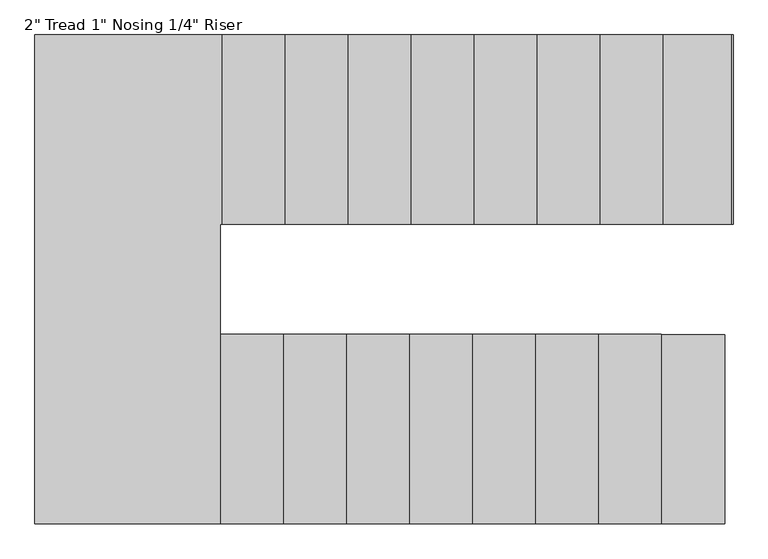
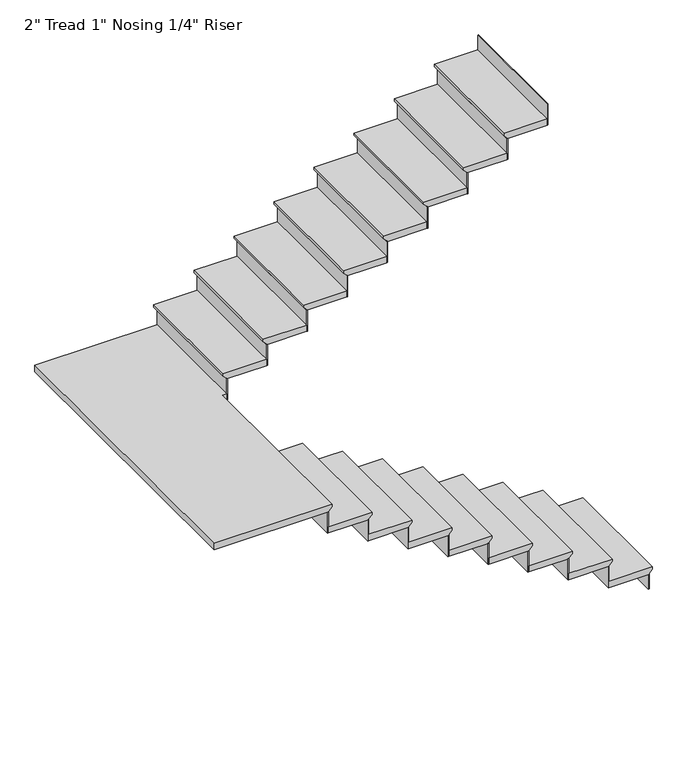
"""IFC4 building model written with IfcOpenShell, lengths in millimetres: stair flight geometry."""

from ifc_helpers import new_model, si_unit, origin, place, context, project, spatial, faceted_brep, source, transform, mapped, element, save


def stair_flight_1ef6648f(model_context):
    return source(origin(), model_context, "Body", "Brep", [
        faceted_brep([(-7930.9736584, -7547.2396616, 455.0833333), (-7930.9736584, -7547.2396616, 474.1333333), (-7930.9736584, -8461.6396616, 474.1333333), (-7930.9736584, -8461.6396616, 455.0833333), (-7956.3736584, -7547.2396616, 429.6833333), (-7956.3736584, -8461.6396616, 429.6833333), (-8261.1736584, -7547.2396616, 474.1333333), (-8261.1736584, -8461.6396616, 474.1333333), (-7956.3736584, -8461.6396616, 423.3333333), (-8261.1736584, -8461.6396616, 423.3333333), (-8261.1736584, -7547.2396616, 423.3333333), (-7956.3736584, -7547.2396616, 423.3333333)], [[[0, 1, 2, 3]], [[4, 0, 3, 5]], [[2, 1, 6, 7]], [[8, 9, 10, 11]], [[2, 7, 9, 8, 5, 3]], [[8, 11, 4, 5]], [[6, 1, 0, 4, 11, 10]], [[7, 6, 10, 9]]]),
        faceted_brep([(-7956.3736584, -7547.2396616, 423.3333333), (-7956.3736584, -7547.2396616, 304.8), (-7962.7236584, -7547.2396616, 304.8), (-7962.7236584, -7547.2396616, 423.3333333), (-7956.3736584, -8461.6396616, 423.3333333), (-7962.7236584, -8461.6396616, 423.3333333), (-7962.7236584, -8461.6396616, 304.8), (-7956.3736584, -8461.6396616, 304.8)], [[[0, 1, 2, 3]], [[4, 5, 6, 7]], [[1, 0, 4, 7]], [[2, 1, 7, 6]], [[3, 2, 6, 5]], [[0, 3, 5, 4]]]),
        faceted_brep([(-8261.1736584, -7547.2396616, 592.6666667), (-8261.1736584, -7547.2396616, 423.3333333), (-8267.5236584, -7547.2396616, 423.3333333), (-8267.5236584, -7547.2396616, 592.6666667), (-8261.1736584, -8461.6396616, 592.6666667), (-8267.5236584, -8461.6396616, 592.6666667), (-8267.5236584, -8461.6396616, 423.3333333), (-8261.1736584, -8461.6396616, 423.3333333)], [[[0, 1, 2, 3]], [[4, 5, 6, 7]], [[1, 0, 4, 7]], [[2, 1, 7, 6]], [[3, 2, 6, 5]], [[0, 3, 5, 4]]]),
        faceted_brep([(-8235.7736584, -8461.6396616, 643.4666667), (-8235.7736584, -7547.2396616, 643.4666667), (-8565.9736584, -7547.2396616, 643.4666667), (-8565.9736584, -8461.6396616, 643.4666667), (-8261.1736584, -8461.6396616, 592.6666667), (-8565.9736584, -8461.6396616, 592.6666667), (-8565.9736584, -7547.2396616, 592.6666667), (-8261.1736584, -7547.2396616, 592.6666667), (-8261.1736584, -8461.6396616, 599.0166667), (-8235.7736584, -8461.6396616, 624.4166667), (-8261.1736584, -7547.2396616, 599.0166667), (-8235.7736584, -7547.2396616, 624.4166667)], [[[0, 1, 2, 3]], [[4, 5, 6, 7]], [[0, 3, 5, 4, 8, 9]], [[4, 7, 10, 8]], [[2, 1, 11, 10, 7, 6]], [[3, 2, 6, 5]], [[11, 1, 0, 9]], [[10, 11, 9, 8]]]),
        faceted_brep([(-8565.9736584, -7547.2396616, 762.0), (-8565.9736584, -7547.2396616, 592.6666667), (-8572.3236584, -7547.2396616, 592.6666667), (-8572.3236584, -7547.2396616, 762.0), (-8565.9736584, -8461.6396616, 762.0), (-8572.3236584, -8461.6396616, 762.0), (-8572.3236584, -8461.6396616, 592.6666667), (-8565.9736584, -8461.6396616, 592.6666667)], [[[0, 1, 2, 3]], [[4, 5, 6, 7]], [[1, 0, 4, 7]], [[2, 1, 7, 6]], [[3, 2, 6, 5]], [[0, 3, 5, 4]]]),
        faceted_brep([(-8540.5736584, -8461.6396616, 812.8), (-8540.5736584, -7547.2396616, 812.8), (-8870.7736584, -7547.2396616, 812.8), (-8870.7736584, -8461.6396616, 812.8), (-8565.9736584, -8461.6396616, 762.0), (-8870.7736584, -8461.6396616, 762.0), (-8870.7736584, -7547.2396616, 762.0), (-8565.9736584, -7547.2396616, 762.0), (-8565.9736584, -8461.6396616, 768.35), (-8540.5736584, -8461.6396616, 793.75), (-8565.9736584, -7547.2396616, 768.35), (-8540.5736584, -7547.2396616, 793.75)], [[[0, 1, 2, 3]], [[4, 5, 6, 7]], [[0, 3, 5, 4, 8, 9]], [[4, 7, 10, 8]], [[2, 1, 11, 10, 7, 6]], [[3, 2, 6, 5]], [[11, 1, 0, 9]], [[10, 11, 9, 8]]]),
        faceted_brep([(-8870.7736584, -7547.2396616, 931.3333333), (-8870.7736584, -7547.2396616, 762.0), (-8877.1236584, -7547.2396616, 762.0), (-8877.1236584, -7547.2396616, 931.3333333), (-8870.7736584, -8461.6396616, 931.3333333), (-8877.1236584, -8461.6396616, 931.3333333), (-8877.1236584, -8461.6396616, 762.0), (-8870.7736584, -8461.6396616, 762.0)], [[[0, 1, 2, 3]], [[4, 5, 6, 7]], [[1, 0, 4, 7]], [[2, 1, 7, 6]], [[3, 2, 6, 5]], [[0, 3, 5, 4]]]),
        faceted_brep([(-8845.3736584, -8461.6396616, 982.1333333), (-8845.3736584, -7547.2396616, 982.1333333), (-9175.5736584, -7547.2396616, 982.1333333), (-9175.5736584, -8461.6396616, 982.1333333), (-8870.7736584, -8461.6396616, 931.3333333), (-9175.5736584, -8461.6396616, 931.3333333), (-9175.5736584, -7547.2396616, 931.3333333), (-8870.7736584, -7547.2396616, 931.3333333), (-8870.7736584, -8461.6396616, 937.6833333), (-8845.3736584, -8461.6396616, 963.0833333), (-8870.7736584, -7547.2396616, 937.6833333), (-8845.3736584, -7547.2396616, 963.0833333)], [[[0, 1, 2, 3]], [[4, 5, 6, 7]], [[0, 3, 5, 4, 8, 9]], [[4, 7, 10, 8]], [[2, 1, 11, 10, 7, 6]], [[3, 2, 6, 5]], [[11, 1, 0, 9]], [[10, 11, 9, 8]]]),
        faceted_brep([(-9175.5736584, -7547.2396616, 1100.6666667), (-9175.5736584, -7547.2396616, 931.3333333), (-9181.9236584, -7547.2396616, 931.3333333), (-9181.9236584, -7547.2396616, 1100.6666667), (-9175.5736584, -8461.6396616, 1100.6666667), (-9181.9236584, -8461.6396616, 1100.6666667), (-9181.9236584, -8461.6396616, 931.3333333), (-9175.5736584, -8461.6396616, 931.3333333)], [[[0, 1, 2, 3]], [[4, 5, 6, 7]], [[1, 0, 4, 7]], [[2, 1, 7, 6]], [[3, 2, 6, 5]], [[0, 3, 5, 4]]]),
        faceted_brep([(-9150.1736584, -8461.6396616, 1151.4666667), (-9150.1736584, -7547.2396616, 1151.4666667), (-9480.3736584, -7547.2396616, 1151.4666667), (-9480.3736584, -8461.6396616, 1151.4666667), (-9175.5736584, -8461.6396616, 1100.6666667), (-9480.3736584, -8461.6396616, 1100.6666667), (-9480.3736584, -7547.2396616, 1100.6666667), (-9175.5736584, -7547.2396616, 1100.6666667), (-9175.5736584, -8461.6396616, 1107.0166667), (-9150.1736584, -8461.6396616, 1132.4166667), (-9175.5736584, -7547.2396616, 1107.0166667), (-9150.1736584, -7547.2396616, 1132.4166667)], [[[0, 1, 2, 3]], [[4, 5, 6, 7]], [[0, 3, 5, 4, 8, 9]], [[4, 7, 10, 8]], [[2, 1, 11, 10, 7, 6]], [[3, 2, 6, 5]], [[11, 1, 0, 9]], [[10, 11, 9, 8]]]),
        faceted_brep([(-9480.3736584, -7547.2396616, 1270.0), (-9480.3736584, -7547.2396616, 1100.6666667), (-9486.7236584, -7547.2396616, 1100.6666667), (-9486.7236584, -7547.2396616, 1270.0), (-9480.3736584, -8461.6396616, 1270.0), (-9486.7236584, -8461.6396616, 1270.0), (-9486.7236584, -8461.6396616, 1100.6666667), (-9480.3736584, -8461.6396616, 1100.6666667)], [[[0, 1, 2, 3]], [[4, 5, 6, 7]], [[1, 0, 4, 7]], [[2, 1, 7, 6]], [[3, 2, 6, 5]], [[0, 3, 5, 4]]]),
        faceted_brep([(-9454.9736584, -8461.6396616, 1320.8), (-9454.9736584, -7547.2396616, 1320.8), (-9785.1736584, -7547.2396616, 1320.8), (-9785.1736584, -8461.6396616, 1320.8), (-9480.3736584, -8461.6396616, 1270.0), (-9785.1736584, -8461.6396616, 1270.0), (-9785.1736584, -7547.2396616, 1270.0), (-9480.3736584, -7547.2396616, 1270.0), (-9480.3736584, -8461.6396616, 1276.35), (-9454.9736584, -8461.6396616, 1301.75), (-9480.3736584, -7547.2396616, 1276.35), (-9454.9736584, -7547.2396616, 1301.75)], [[[0, 1, 2, 3]], [[4, 5, 6, 7]], [[0, 3, 5, 4, 8, 9]], [[4, 7, 10, 8]], [[2, 1, 11, 10, 7, 6]], [[3, 2, 6, 5]], [[11, 1, 0, 9]], [[10, 11, 9, 8]]]),
        faceted_brep([(-9785.1736584, -7547.2396616, 1439.3333333), (-9785.1736584, -7547.2396616, 1270.0), (-9791.5236584, -7547.2396616, 1270.0), (-9791.5236584, -7547.2396616, 1439.3333333), (-9785.1736584, -8461.6396616, 1439.3333333), (-9791.5236584, -8461.6396616, 1439.3333333), (-9791.5236584, -8461.6396616, 1270.0), (-9785.1736584, -8461.6396616, 1270.0)], [[[0, 1, 2, 3]], [[4, 5, 6, 7]], [[1, 0, 4, 7]], [[2, 1, 7, 6]], [[3, 2, 6, 5]], [[0, 3, 5, 4]]]),
        faceted_brep([(-9759.7736584, -8461.6396616, 1490.1333333), (-9759.7736584, -7547.2396616, 1490.1333333), (-10089.9736584, -7547.2396616, 1490.1333333), (-10089.9736584, -8461.6396616, 1490.1333333), (-9785.1736584, -8461.6396616, 1439.3333333), (-10089.9736584, -8461.6396616, 1439.3333333), (-10089.9736584, -7547.2396616, 1439.3333333), (-9785.1736584, -7547.2396616, 1439.3333333), (-9785.1736584, -8461.6396616, 1445.6833333), (-9759.7736584, -8461.6396616, 1471.0833333), (-9785.1736584, -7547.2396616, 1445.6833333), (-9759.7736584, -7547.2396616, 1471.0833333)], [[[0, 1, 2, 3]], [[4, 5, 6, 7]], [[0, 3, 5, 4, 8, 9]], [[4, 7, 10, 8]], [[2, 1, 11, 10, 7, 6]], [[3, 2, 6, 5]], [[11, 1, 0, 9]], [[10, 11, 9, 8]]]),
        faceted_brep([(-10089.9736584, -7547.2396616, 1608.6666667), (-10089.9736584, -7547.2396616, 1439.3333333), (-10096.3236584, -7547.2396616, 1439.3333333), (-10096.3236584, -7547.2396616, 1608.6666667), (-10089.9736584, -8461.6396616, 1608.6666667), (-10096.3236584, -8461.6396616, 1608.6666667), (-10096.3236584, -8461.6396616, 1439.3333333), (-10089.9736584, -8461.6396616, 1439.3333333)], [[[0, 1, 2, 3]], [[4, 5, 6, 7]], [[1, 0, 4, 7]], [[2, 1, 7, 6]], [[3, 2, 6, 5]], [[0, 3, 5, 4]]]),
        faceted_brep([(-10064.5736584, -8461.6396616, 1659.4666667), (-10064.5736584, -7547.2396616, 1659.4666667), (-10394.7736584, -7547.2396616, 1659.4666667), (-10394.7736584, -8461.6396616, 1659.4666667), (-10089.9736584, -8461.6396616, 1608.6666667), (-10394.7736584, -8461.6396616, 1608.6666667), (-10394.7736584, -7547.2396616, 1608.6666667), (-10089.9736584, -7547.2396616, 1608.6666667), (-10089.9736584, -8461.6396616, 1615.0166667), (-10064.5736584, -8461.6396616, 1640.4166667), (-10089.9736584, -7547.2396616, 1615.0166667), (-10064.5736584, -7547.2396616, 1640.4166667)], [[[0, 1, 2, 3]], [[4, 5, 6, 7]], [[0, 3, 5, 4, 8, 9]], [[4, 7, 10, 8]], [[2, 1, 11, 10, 7, 6]], [[3, 2, 6, 5]], [[11, 1, 0, 9]], [[10, 11, 9, 8]]]),
        faceted_brep([(-10394.7736584, -7547.2396616, 1778.0), (-10394.7736584, -7547.2396616, 1608.6666667), (-10401.1236584, -7547.2396616, 1608.6666667), (-10401.1236584, -7547.2396616, 1778.0), (-10394.7736584, -8461.6396616, 1778.0), (-10401.1236584, -8461.6396616, 1778.0), (-10401.1236584, -8461.6396616, 1608.6666667), (-10394.7736584, -8461.6396616, 1608.6666667)], [[[0, 1, 2, 3]], [[4, 5, 6, 7]], [[1, 0, 4, 7]], [[2, 1, 7, 6]], [[3, 2, 6, 5]], [[0, 3, 5, 4]]]),
        faceted_brep([(-10334.3270642, -6099.4396616, 1828.8), (-11264.7236584, -6099.4396616, 1828.8), (-11264.7236584, -8461.6396616, 1828.8), (-10369.3736584, -8461.6396616, 1828.8), (-10369.3736584, -7013.8396616, 1828.8), (-10334.3270642, -7013.8396616, 1828.8), (-11264.7236584, -6099.4396616, 1778.0), (-10334.3270642, -6099.4396616, 1778.0), (-10334.3270642, -7013.8396616, 1778.0), (-10369.3736584, -7013.8396616, 1778.0), (-10369.3736584, -7547.2396616, 1778.0), (-10394.7736584, -7547.2396616, 1778.0), (-10394.7736584, -8461.6396616, 1778.0), (-11264.7236584, -8461.6396616, 1778.0), (-10394.7736584, -8461.6396616, 1784.35), (-10369.3736584, -8461.6396616, 1809.75), (-10394.7736584, -7547.2396616, 1784.35), (-10369.3736584, -7547.2396616, 1809.75)], [[[0, 1, 2, 3, 4, 5]], [[6, 7, 8, 9, 10, 11, 12, 13]], [[1, 0, 7, 6]], [[2, 1, 6, 13]], [[3, 2, 13, 12, 14, 15]], [[12, 11, 16, 14]], [[11, 10, 17, 16]], [[4, 3, 15, 17, 10, 9]], [[5, 4, 9, 8]], [[0, 5, 8, 7]], [[15, 14, 16, 17]]]),
        faceted_brep([(-10334.3270642, -7013.8396616, 1947.3333333), (-10334.3270642, -7013.8396616, 1778.0), (-10327.9770642, -7013.8396616, 1778.0), (-10327.9770642, -7013.8396616, 1947.3333333), (-10334.3270642, -6099.4396616, 1947.3333333), (-10327.9770642, -6099.4396616, 1947.3333333), (-10327.9770642, -6099.4396616, 1778.0), (-10334.3270642, -6099.4396616, 1778.0)], [[[0, 1, 2, 3]], [[4, 5, 6, 7]], [[1, 0, 4, 7]], [[2, 1, 7, 6]], [[3, 2, 6, 5]], [[0, 3, 5, 4]]]),
        faceted_brep([(-10359.7270642, -6099.4396616, 1998.1333333), (-10359.7270642, -7013.8396616, 1998.1333333), (-10029.5270642, -7013.8396616, 1998.1333333), (-10029.5270642, -6099.4396616, 1998.1333333), (-10334.3270642, -6099.4396616, 1947.3333333), (-10029.5270642, -6099.4396616, 1947.3333333), (-10029.5270642, -7013.8396616, 1947.3333333), (-10334.3270642, -7013.8396616, 1947.3333333), (-10334.3270642, -6099.4396616, 1953.6833333), (-10359.7270642, -6099.4396616, 1979.0833333), (-10334.3270642, -7013.8396616, 1953.6833333), (-10359.7270642, -7013.8396616, 1979.0833333)], [[[0, 1, 2, 3]], [[4, 5, 6, 7]], [[0, 3, 5, 4, 8, 9]], [[4, 7, 10, 8]], [[2, 1, 11, 10, 7, 6]], [[3, 2, 6, 5]], [[11, 1, 0, 9]], [[10, 11, 9, 8]]]),
        faceted_brep([(-10029.5270642, -7013.8396616, 2116.6666667), (-10029.5270642, -7013.8396616, 1947.3333333), (-10023.1770642, -7013.8396616, 1947.3333333), (-10023.1770642, -7013.8396616, 2116.6666667), (-10029.5270642, -6099.4396616, 2116.6666667), (-10023.1770642, -6099.4396616, 2116.6666667), (-10023.1770642, -6099.4396616, 1947.3333333), (-10029.5270642, -6099.4396616, 1947.3333333)], [[[0, 1, 2, 3]], [[4, 5, 6, 7]], [[1, 0, 4, 7]], [[2, 1, 7, 6]], [[3, 2, 6, 5]], [[0, 3, 5, 4]]]),
        faceted_brep([(-10054.9270642, -6099.4396616, 2167.4666667), (-10054.9270642, -7013.8396616, 2167.4666667), (-9724.7270642, -7013.8396616, 2167.4666667), (-9724.7270642, -6099.4396616, 2167.4666667), (-10029.5270642, -6099.4396616, 2116.6666667), (-9724.7270642, -6099.4396616, 2116.6666667), (-9724.7270642, -7013.8396616, 2116.6666667), (-10029.5270642, -7013.8396616, 2116.6666667), (-10029.5270642, -6099.4396616, 2123.0166667), (-10054.9270642, -6099.4396616, 2148.4166667), (-10029.5270642, -7013.8396616, 2123.0166667), (-10054.9270642, -7013.8396616, 2148.4166667)], [[[0, 1, 2, 3]], [[4, 5, 6, 7]], [[0, 3, 5, 4, 8, 9]], [[4, 7, 10, 8]], [[2, 1, 11, 10, 7, 6]], [[3, 2, 6, 5]], [[11, 1, 0, 9]], [[10, 11, 9, 8]]]),
        faceted_brep([(-9724.7270642, -7013.8396616, 2286.0), (-9724.7270642, -7013.8396616, 2116.6666667), (-9718.3770642, -7013.8396616, 2116.6666667), (-9718.3770642, -7013.8396616, 2286.0), (-9724.7270642, -6099.4396616, 2286.0), (-9718.3770642, -6099.4396616, 2286.0), (-9718.3770642, -6099.4396616, 2116.6666667), (-9724.7270642, -6099.4396616, 2116.6666667)], [[[0, 1, 2, 3]], [[4, 5, 6, 7]], [[1, 0, 4, 7]], [[2, 1, 7, 6]], [[3, 2, 6, 5]], [[0, 3, 5, 4]]]),
        faceted_brep([(-9750.1270642, -6099.4396616, 2336.8), (-9750.1270642, -7013.8396616, 2336.8), (-9419.9270642, -7013.8396616, 2336.8), (-9419.9270642, -6099.4396616, 2336.8), (-9724.7270642, -6099.4396616, 2286.0), (-9419.9270642, -6099.4396616, 2286.0), (-9419.9270642, -7013.8396616, 2286.0), (-9724.7270642, -7013.8396616, 2286.0), (-9724.7270642, -6099.4396616, 2292.35), (-9750.1270642, -6099.4396616, 2317.75), (-9724.7270642, -7013.8396616, 2292.35), (-9750.1270642, -7013.8396616, 2317.75)], [[[0, 1, 2, 3]], [[4, 5, 6, 7]], [[0, 3, 5, 4, 8, 9]], [[4, 7, 10, 8]], [[2, 1, 11, 10, 7, 6]], [[3, 2, 6, 5]], [[11, 1, 0, 9]], [[10, 11, 9, 8]]]),
        faceted_brep([(-9419.9270642, -7013.8396616, 2455.3333333), (-9419.9270642, -7013.8396616, 2286.0), (-9413.5770642, -7013.8396616, 2286.0), (-9413.5770642, -7013.8396616, 2455.3333333), (-9419.9270642, -6099.4396616, 2455.3333333), (-9413.5770642, -6099.4396616, 2455.3333333), (-9413.5770642, -6099.4396616, 2286.0), (-9419.9270642, -6099.4396616, 2286.0)], [[[0, 1, 2, 3]], [[4, 5, 6, 7]], [[1, 0, 4, 7]], [[2, 1, 7, 6]], [[3, 2, 6, 5]], [[0, 3, 5, 4]]]),
        faceted_brep([(-9445.3270642, -6099.4396616, 2506.1333333), (-9445.3270642, -7013.8396616, 2506.1333333), (-9115.1270642, -7013.8396616, 2506.1333333), (-9115.1270642, -6099.4396616, 2506.1333333), (-9419.9270642, -6099.4396616, 2455.3333333), (-9115.1270642, -6099.4396616, 2455.3333333), (-9115.1270642, -7013.8396616, 2455.3333333), (-9419.9270642, -7013.8396616, 2455.3333333), (-9419.9270642, -6099.4396616, 2461.6833333), (-9445.3270642, -6099.4396616, 2487.0833333), (-9419.9270642, -7013.8396616, 2461.6833333), (-9445.3270642, -7013.8396616, 2487.0833333)], [[[0, 1, 2, 3]], [[4, 5, 6, 7]], [[0, 3, 5, 4, 8, 9]], [[4, 7, 10, 8]], [[2, 1, 11, 10, 7, 6]], [[3, 2, 6, 5]], [[11, 1, 0, 9]], [[10, 11, 9, 8]]]),
        faceted_brep([(-9115.1270642, -7013.8396616, 2624.6666667), (-9115.1270642, -7013.8396616, 2455.3333333), (-9108.7770642, -7013.8396616, 2455.3333333), (-9108.7770642, -7013.8396616, 2624.6666667), (-9115.1270642, -6099.4396616, 2624.6666667), (-9108.7770642, -6099.4396616, 2624.6666667), (-9108.7770642, -6099.4396616, 2455.3333333), (-9115.1270642, -6099.4396616, 2455.3333333)], [[[0, 1, 2, 3]], [[4, 5, 6, 7]], [[1, 0, 4, 7]], [[2, 1, 7, 6]], [[3, 2, 6, 5]], [[0, 3, 5, 4]]]),
        faceted_brep([(-9140.5270642, -6099.4396616, 2675.4666667), (-9140.5270642, -7013.8396616, 2675.4666667), (-8810.3270642, -7013.8396616, 2675.4666667), (-8810.3270642, -6099.4396616, 2675.4666667), (-9115.1270642, -6099.4396616, 2624.6666667), (-8810.3270642, -6099.4396616, 2624.6666667), (-8810.3270642, -7013.8396616, 2624.6666667), (-9115.1270642, -7013.8396616, 2624.6666667), (-9115.1270642, -6099.4396616, 2631.0166667), (-9140.5270642, -6099.4396616, 2656.4166667), (-9115.1270642, -7013.8396616, 2631.0166667), (-9140.5270642, -7013.8396616, 2656.4166667)], [[[0, 1, 2, 3]], [[4, 5, 6, 7]], [[0, 3, 5, 4, 8, 9]], [[4, 7, 10, 8]], [[2, 1, 11, 10, 7, 6]], [[3, 2, 6, 5]], [[11, 1, 0, 9]], [[10, 11, 9, 8]]]),
        faceted_brep([(-8810.3270642, -7013.8396616, 2794.0), (-8810.3270642, -7013.8396616, 2624.6666667), (-8803.9770642, -7013.8396616, 2624.6666667), (-8803.9770642, -7013.8396616, 2794.0), (-8810.3270642, -6099.4396616, 2794.0), (-8803.9770642, -6099.4396616, 2794.0), (-8803.9770642, -6099.4396616, 2624.6666667), (-8810.3270642, -6099.4396616, 2624.6666667)], [[[0, 1, 2, 3]], [[4, 5, 6, 7]], [[1, 0, 4, 7]], [[2, 1, 7, 6]], [[3, 2, 6, 5]], [[0, 3, 5, 4]]]),
        faceted_brep([(-8835.7270642, -6099.4396616, 2844.8), (-8835.7270642, -7013.8396616, 2844.8), (-8505.5270642, -7013.8396616, 2844.8), (-8505.5270642, -6099.4396616, 2844.8), (-8810.3270642, -6099.4396616, 2794.0), (-8505.5270642, -6099.4396616, 2794.0), (-8505.5270642, -7013.8396616, 2794.0), (-8810.3270642, -7013.8396616, 2794.0), (-8810.3270642, -6099.4396616, 2800.35), (-8835.7270642, -6099.4396616, 2825.75), (-8810.3270642, -7013.8396616, 2800.35), (-8835.7270642, -7013.8396616, 2825.75)], [[[0, 1, 2, 3]], [[4, 5, 6, 7]], [[0, 3, 5, 4, 8, 9]], [[4, 7, 10, 8]], [[2, 1, 11, 10, 7, 6]], [[3, 2, 6, 5]], [[11, 1, 0, 9]], [[10, 11, 9, 8]]]),
        faceted_brep([(-8505.5270642, -7013.8396616, 2963.3333333), (-8505.5270642, -7013.8396616, 2794.0), (-8499.1770642, -7013.8396616, 2794.0), (-8499.1770642, -7013.8396616, 2963.3333333), (-8505.5270642, -6099.4396616, 2963.3333333), (-8499.1770642, -6099.4396616, 2963.3333333), (-8499.1770642, -6099.4396616, 2794.0), (-8505.5270642, -6099.4396616, 2794.0)], [[[0, 1, 2, 3]], [[4, 5, 6, 7]], [[1, 0, 4, 7]], [[2, 1, 7, 6]], [[3, 2, 6, 5]], [[0, 3, 5, 4]]]),
        faceted_brep([(-8530.9270642, -6099.4396616, 3014.1333333), (-8530.9270642, -7013.8396616, 3014.1333333), (-8200.7270642, -7013.8396616, 3014.1333333), (-8200.7270642, -6099.4396616, 3014.1333333), (-8505.5270642, -6099.4396616, 2963.3333333), (-8200.7270642, -6099.4396616, 2963.3333333), (-8200.7270642, -7013.8396616, 2963.3333333), (-8505.5270642, -7013.8396616, 2963.3333333), (-8505.5270642, -6099.4396616, 2969.6833333), (-8530.9270642, -6099.4396616, 2995.0833333), (-8505.5270642, -7013.8396616, 2969.6833333), (-8530.9270642, -7013.8396616, 2995.0833333)], [[[0, 1, 2, 3]], [[4, 5, 6, 7]], [[0, 3, 5, 4, 8, 9]], [[4, 7, 10, 8]], [[2, 1, 11, 10, 7, 6]], [[3, 2, 6, 5]], [[11, 1, 0, 9]], [[10, 11, 9, 8]]]),
        faceted_brep([(-8200.7270642, -7013.8396616, 3132.6666667), (-8200.7270642, -7013.8396616, 2963.3333333), (-8194.3770642, -7013.8396616, 2963.3333333), (-8194.3770642, -7013.8396616, 3132.6666667), (-8200.7270642, -6099.4396616, 3132.6666667), (-8194.3770642, -6099.4396616, 3132.6666667), (-8194.3770642, -6099.4396616, 2963.3333333), (-8200.7270642, -6099.4396616, 2963.3333333)], [[[0, 1, 2, 3]], [[4, 5, 6, 7]], [[1, 0, 4, 7]], [[2, 1, 7, 6]], [[3, 2, 6, 5]], [[0, 3, 5, 4]]]),
        faceted_brep([(-7895.9270642, -7013.8396616, 3302.0), (-7895.9270642, -7013.8396616, 3132.6666667), (-7889.5770642, -7013.8396616, 3132.6666667), (-7889.5770642, -7013.8396616, 3302.0), (-7895.9270642, -6099.4396616, 3302.0), (-7889.5770642, -6099.4396616, 3302.0), (-7889.5770642, -6099.4396616, 3132.6666667), (-7895.9270642, -6099.4396616, 3132.6666667)], [[[0, 1, 2, 3]], [[4, 5, 6, 7]], [[1, 0, 4, 7]], [[2, 1, 7, 6]], [[3, 2, 6, 5]], [[0, 3, 5, 4]]]),
        faceted_brep([(-8226.1270642, -6099.4396616, 3183.4666667), (-8226.1270642, -7013.8396616, 3183.4666667), (-7895.9270642, -7013.8396616, 3183.4666667), (-7895.9270642, -6099.4396616, 3183.4666667), (-8200.7270642, -6099.4396616, 3132.6666667), (-7895.9270642, -6099.4396616, 3132.6666667), (-7895.9270642, -7013.8396616, 3132.6666667), (-8200.7270642, -7013.8396616, 3132.6666667), (-8200.7270642, -6099.4396616, 3139.0166667), (-8226.1270642, -6099.4396616, 3164.4166667), (-8200.7270642, -7013.8396616, 3139.0166667), (-8226.1270642, -7013.8396616, 3164.4166667)], [[[0, 1, 2, 3]], [[4, 5, 6, 7]], [[0, 3, 5, 4, 8, 9]], [[4, 7, 10, 8]], [[2, 1, 11, 10, 7, 6]], [[3, 2, 6, 5]], [[11, 1, 0, 9]], [[10, 11, 9, 8]]]),
    ])


if __name__ == "__main__":
    model = new_model("IFC4")
    model_context = context("Model", 3, world=origin())
    ifc_project = project(units=[si_unit("LENGTHUNIT", "METRE", prefix="MILLI")], contexts=[model_context])
    site = spatial("IfcSite", under=ifc_project)
    building = spatial("IfcBuilding", under=site)
    placement = place(None, origin())
    stair_flight_shape = stair_flight_1ef6648f(model_context)
    element("IfcStairFlight", 1, ObjectType="2\" Tread 1\" Nosing 1/4\" Riser", at=placement, inside=building, context=model_context, shape_type="MappedRepresentation", body=[
        mapped(stair_flight_shape, transform((0.0, 0.0, 0.0), x_axis=(1.0, 0.0, 0.0), y_axis=(0.0, 1.0, 0.0), z_axis=(0.0, 0.0, 1.0))),
    ])
    save(model, "model.ifc")

# Revit data of these elements
# Element 1 (IfcStairFlight, "2\" Tread 1\" Nosing 1/4\" Riser")
#   Materials on its faces: "MARBLE FLOORING 6\""
# Materials
#   "MARBLE FLOORING 6\"": class "Generic", colour RGB 120 120 120, transparency 0, Cost = 0
